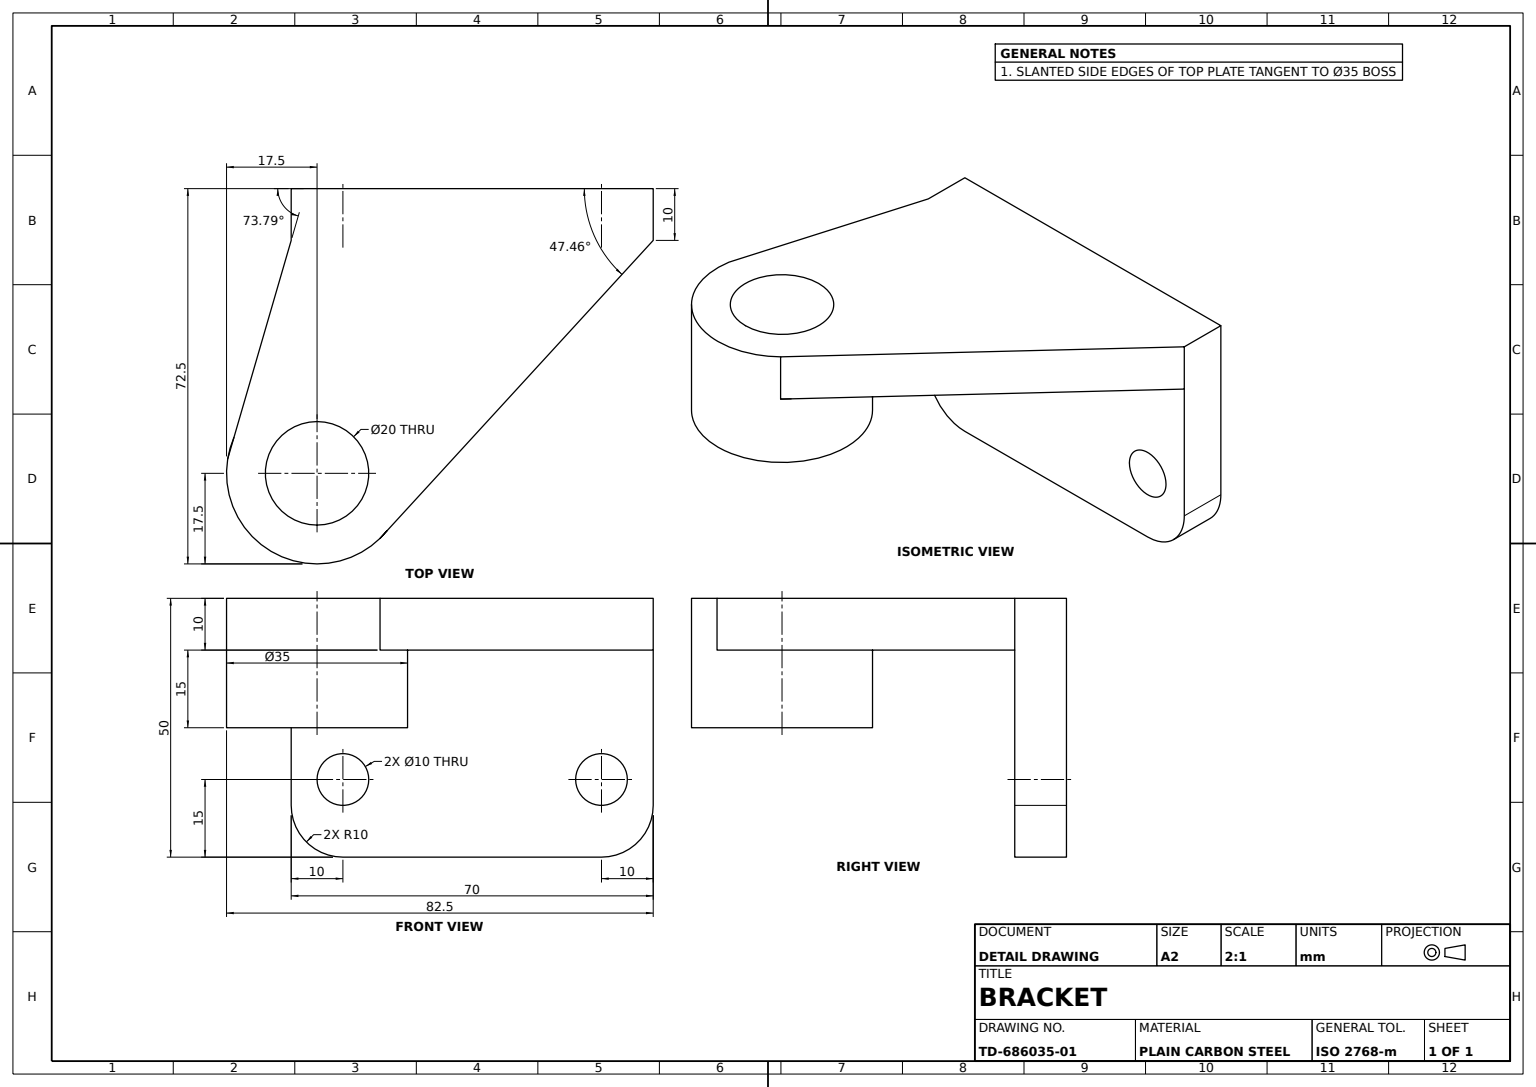
from build123d import *

# Parameters (mm, degrees)
BASE_PLATE_DEPTH         = 10
SIDE_PLATE_DEPTH         = 10
HUB_BOSS_SKETCH_R        = 17.5
HUB_BOSS_35_DEPTH        = 15
HUB_BORE_SKETCH_R        = 10
HUB_BORE_20_DEPTH        = 25
SIDE_PLATE_HOLE_SKETCH_R = 5
SIDE_PLATE_HOLE_DEPTH    = 10


with BuildPart() as part:
    # Base Plate Sketch → Base Plate (new body)
    with BuildSketch(Plane.XY):
        with BuildLine():
            Line((0, 0), (0, -40))
            ThreePointArc((0, -40), (2.928932188, -47.071067812), (10, -50))
            Line((10, -50), (60, -50))
            ThreePointArc((60, -50), (67.071067812, -47.071067812), (70, -40))
            Line((70, -40), (70, 0))
            Line((70, 0), (0, 0))
        make_face()
    extrude(amount=BASE_PLATE_DEPTH)

    # Side Plate Sketch → Side Plate (add)
    with BuildSketch(Plane(origin=(0, 0, 0), x_dir=(1, 0, 0), z_dir=(0, 1, 0))):
        with BuildLine():
            Line((18.565158101, -66.056061039), (70, -10))
            Line((70, -10), (0, -10))
            Line((0, -10), (-11.072048142, -48.076181073))
            ThreePointArc((-11.072048142, -48.076181073), (8.534767144, -37.860705346), (22.5, -55))
            ThreePointArc((22.5, -55), (21.486968593, -60.867696875), (18.565158101, -66.056061039))
        make_face()
        with BuildLine():
            Line((17.179494078, -67.566221548), (18.565158101, -66.056061039))
            ThreePointArc((18.565158101, -66.056061039), (21.486968593, -60.867696875), (22.5, -55))
            ThreePointArc((22.5, -55), (8.534767144, -37.860705346), (-11.072048142, -48.076181073))
            Line((-11.072048142, -48.076181073), (-12.278719231, -52.225858378))
            ThreePointArc((-12.278719231, -52.225858378), (-3.08283427, -70.52152667), (17.179494078, -67.566221548))
        make_face()
    extrude(amount=-SIDE_PLATE_DEPTH)

    # Hub Boss Sketch → Hub Boss Ø35 (add)
    with BuildSketch(Plane.XZ.offset(10)):
        with Locations(Location((5, 55, 0), (0, 0, 45.895348857))):
            Circle(HUB_BOSS_SKETCH_R)
    extrude(amount=HUB_BOSS_35_DEPTH)

    # Hub Bore Sketch → Hub Bore Ø20 (cut)
    with BuildSketch(Plane.XZ.offset(25)):
        with Locations(Location((5, 55, 0), (0, 0, 270))):
            Circle(HUB_BORE_SKETCH_R)
    extrude(amount=-HUB_BORE_20_DEPTH, mode=Mode.SUBTRACT)

    # Side Plate Hole Sketch → Side Plate Hole (cut)
    with BuildSketch(Plane.XY.offset(10)):
        with Locations((10, -35)):
            Circle(SIDE_PLATE_HOLE_SKETCH_R)
        with Locations((60, -35)):
            Circle(SIDE_PLATE_HOLE_SKETCH_R)
    extrude(amount=-SIDE_PLATE_HOLE_DEPTH, mode=Mode.SUBTRACT)


solid = part.part
